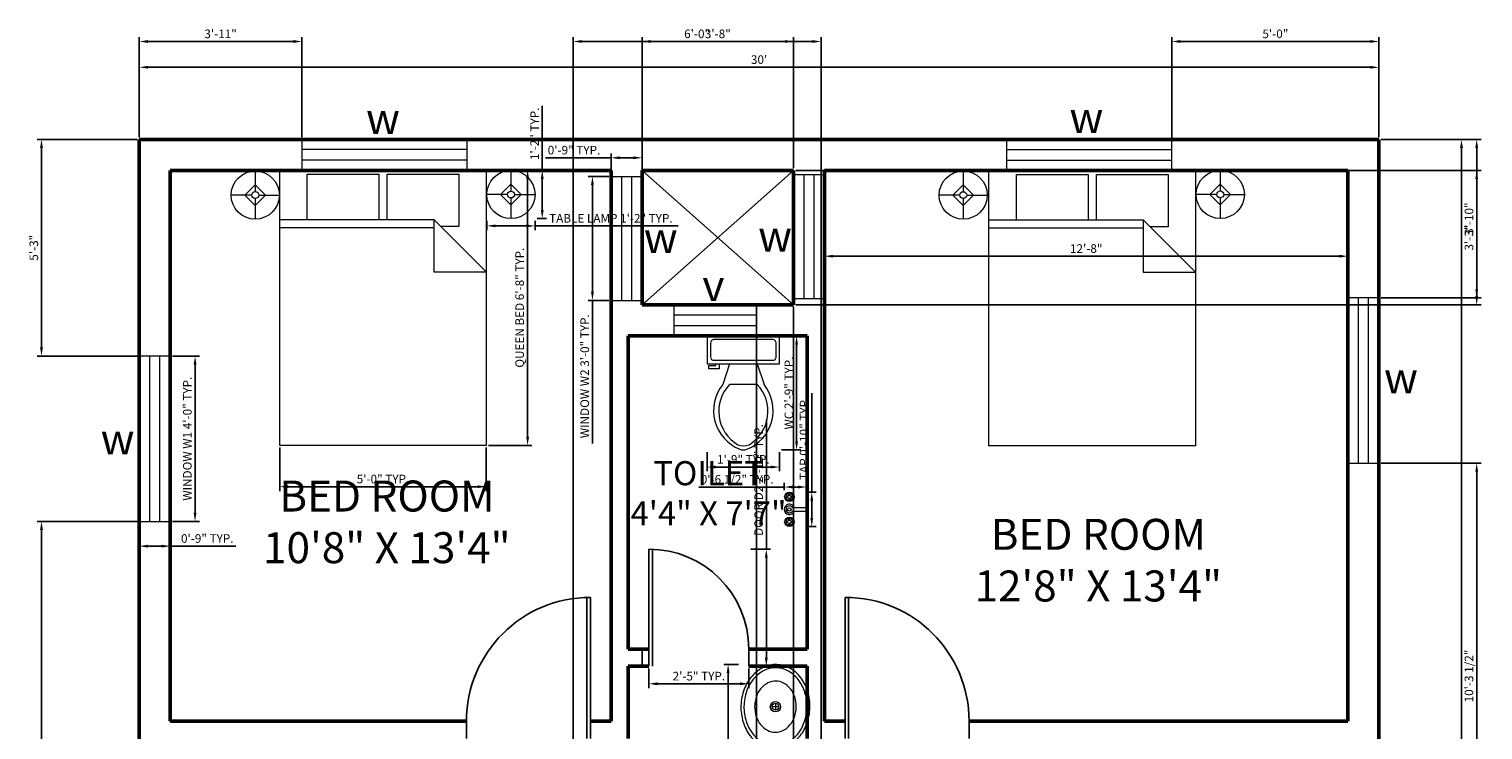
# Model space of a CAD drawing. Units: inches. Extents: x 1962 to 2423, y 2693 to 3296.
# Tile 4 of 4: x 1965 to 2387, y 3092 to 3296. Entities that reach past the tile are written whole.
import ezdxf

# ---------------------------------------------------------------- set-up
doc = ezdxf.new("R2010")
doc.units = ezdxf.units.IN
for name, color, linetype, lineweight in [('A-ANNO-DIMS', 2, 'Continuous', 18), ('A-ANNO-SYMB', 7, 'Continuous', 18), ('A-ANNO-TEXT', 3, 'Continuous', 18), ('A-AREA-IDEN', 7, 'Continuous', 25), ('A-DOOR', 3, 'Continuous', 25), ('A-FLOR-FIXT', 9, 'Continuous', 18), ('A-FURN', 8, 'Continuous', 18), ('A-GLAZ', 4, 'Continuous', 18), ('A-WALL', 7, 'Continuous', 50)]:
    doc.layers.add(name, color=color, linetype=linetype, lineweight=lineweight)
doc.styles.get("Standard").update_dxf_attribs({"font": 'arial.ttf'})
doc.dimstyles.new('ISO-25', dxfattribs={"dimtxt": 2.5, "dimasz": 2.5, "dimexe": 1.25, "dimexo": 0.625, "dimtad": 1, "dimdec": 0, "dimlunit": 3, "dimtxsty": 'Standard', "dimcen": 2.5, "dimadec": 0, "dimazin": 0, "dimtfac": 1, "dimtdec": 0, "dimtmove": 0, "dimatfit": 3, "dimfxl": 1, "dimarcsym": 0})

# ---------------------------------------------------------------- blocks, each defined once
blk = doc.blocks.new('Bed - Queen')
for p, q in [((0, -80.00003), (0, 0)), ((0, 0), (59.99999, 0)), ((59.99999, 0), (59.99999, -80.00003)), ((7.99999, -1.2), (28.79998, -1.2)), ((7.99999, -14.4), (7.99999, -1.2)), ((28.79998, -1.2), (28.79998, -14.4)), ((31.19999, -1.2), (51.99999, -1.2)), ((31.19999, -14.4), (31.19999, -1.2)), ((51.99999, -1.2), (51.99999, -16.4)), ((0, -14.4), (44.8, -14.4)), ((44.8, -16.8), (0, -16.8)), ((59.99999, -29.6), (44.8, -14.4)), ((44.8, -14.4), (44.8, -29.6)), ((51.99999, -16.4), (46.79936, -16.4)), ((44.8, -29.6), (59.99999, -29.6)), ((59.99999, -80.00003), (0, -80.00003))]:
    blk.add_line(p, q)
blk = doc.blocks.new('Lamp - Table')
for p, q in [((0, 7), (0, 1)), ((-1, 0), (-7, 0)), ((0, 3), (-3, 0)), ((-3, 0), (0, -3)), ((3, 0), (0, 3)), ((0, -3), (3, 0)), ((1, 0), (7, 0)), ((0, -1), (0, -7))]:
    blk.add_line(p, q)
for radius in [7, 1]:
    blk.add_circle((0, 0), radius)
blk = doc.blocks.new('Sink - Oval top')
for p, q in [((-1, 0), (1, 0)), ((0, 1), (0, -1))]:
    blk.add_line(p, q)
for points in [[(-12.23, 0.39, 0.117634), (-11.46, -3.36, 0.104469), (-8.88, -6.8, 0.090016), (-5.08, -9.07, 0.08192), (-0.32, -10.02, 0.08192), (4.49, -9.38, 0.090016), (8.42, -7.36, 0.104469), (11.22, -4.09, 0.117634), (12.23, -0.39, 0.117634), (11.46, 3.36, 0.104469), (8.88, 6.8, 0.090016), (5.08, 9.07, 0.08192), (0.32, 10.02, 0.08192), (-4.49, 9.38, 0.090016), (-8.42, 7.36, 0.104469), (-11.22, 4.09, 0.117634)], [(-11.29, 0.16, 0.118622), (-10.52, -3.25, 0.104678), (-8.07, -6.36, 0.089562), (-4.54, -8.37, 0.081185), (-0.13, -9.15, 0.081185), (4.3, -8.49, 0.089562), (7.89, -6.58, 0.104678), (10.42, -3.55, 0.118622), (11.29, -0.16, 0.118622), (10.52, 3.25, 0.104678), (8.07, 6.36, 0.089562), (4.54, 8.37, 0.081185), (0.13, 9.15, 0.081185), (-4.3, 8.49, 0.089562), (-7.89, 6.58, 0.104678), (-10.42, 3.55, 0.118622)], [(-7.42, 0.08, 0.118283), (-6.91, -2.17, 0.104607), (-5.29, -4.21, 0.089718), (-2.97, -5.53, 0.081436), (-0.07, -6.04, 0.081436), (2.84, -5.59, 0.089718), (5.2, -4.33, 0.104607), (6.86, -2.32, 0.118283), (7.42, -0.08, 0.118283), (6.91, 2.17, 0.104607), (5.29, 4.21, 0.089718), (2.97, 5.53, 0.081436), (0.07, 6.04, 0.081436), (-2.84, 5.59, 0.089718), (-5.2, 4.33, 0.104607), (-6.86, 2.32, 0.118283)]]:
    blk.add_lwpolyline(points, format="xyb", close=True)
for radius in [1.5, 1]:
    blk.add_circle((0, 0), radius)
blk = doc.blocks.new('Toilet - top')
for p, q in [((9.5, -6), (9.5, -2)), ((-8, -8.5), (-8, -8)), ((-7, -8), (-7, -9.5)), ((-4, -8), (-6, -14)), ((4, -8), (6, -14)), ((-10, -8.5), (-8, -8.5)), ((-10, -9.5), (-10, -8.5)), ((-7, -9.5), (-10, -9.5)), ((4, -14), (-4, -14))]:
    blk.add_line(p, q)
blk.add_lwpolyline([(10.5, -8), (10.5, 0), (-10.5, 0), (-10.5, -8)], close=True)
for points in [[(-9.5, -2), (-9.5, -6)], [(8.5, -1), (-8.5, -1)], [(-8.5, -7), (8.5, -7)]]:
    blk.add_lwpolyline(points)
for centre, radius, start, end in [((-8.62, -1.88), 0.884, 81.8699, 188.1301), ((8.62, -1.88), 0.884, 351.8699, 98.1301), ((-8.62, -6.12), 0.884, 171.8699, 278.1301), ((8.62, -6.12), 0.884, 261.8699, 8.1301), ((3.52, -21.58), 12.17, 141.4691, 247.9714), ((4.2, -21.82), 11.33, 136.3677, 238.9468), ((-3.52, -21.58), 12.17, 292.0284, 38.5307), ((-4.2, -21.82), 11.33, 301.053, 43.6321), ((0, -27.88), 4, 245.7318, 294.2682), ((0, -29), 4, 254.8605, 285.1395)]:
    blk.add_arc(centre, radius, start, end)
blk = doc.blocks.new('Faucet - Bathroom top')
for p, q in [((-4.107, 0.125), (-4.375, 0.125)), ((-3.75, 0.4788), (-3.75, 0.75)), ((-3.5, 0.482), (-3.5, 0.75)), ((-3.1461, 0.125), (-2.875, 0.125)), ((3.143, 0.125), (2.875, 0.125)), ((3.5, 0.4788), (3.5, 0.75)), ((3.75, 0.482), (3.75, 0.75)), ((4.1039, 0.125), (4.375, 0.125)), ((-4.1039, -0.125), (-4.375, -0.125)), ((-3.75, -0.4821), (-3.75, -0.75)), ((-3.5, -0.4789), (-3.5, -0.75)), ((-3.143, -0.125), (-2.875, -0.125)), ((-0.5, -0.8639), (-0.5, -4.5)), ((0.5, -4.5), (0.5, -0.8631)), ((3.1461, -0.125), (2.875, -0.125)), ((3.5, -0.4821), (3.5, -0.75)), ((3.75, -0.4789), (3.75, -0.75)), ((4.107, -0.125), (4.375, -0.125))]:
    blk.add_line(p, q)
for centre, radius in [((-3.625, 0), 1.375), ((-4.625, 0), 0.2795), ((-3.625, 0), 0.5), ((-3.625, 1), 0.2795), ((-2.625, 0), 0.2795), ((0, 0), 0.5), ((3.625, 0), 1.375), ((2.625, 0), 0.2795), ((3.625, 0), 0.5), ((3.625, 1), 0.2795), ((4.625, 0), 0.2795), ((-3.625, -1), 0.2795), ((3.625, -1), 0.2795)]:
    blk.add_circle(centre, radius)
for centre, radius, start, end in [((-3.625, 0), 1, 105.2407, 164.2093), ((-3.625, 0), 1, 16.44125, 74.07887), ((0, 0), 1.5, 289.6514, 250.3603), ((0, 0), 1, 300.3431, 239.7554), ((3.625, 0), 1, 106.12, 164.0884), ((3.625, 0), 1, 16.23422, 73.90469), ((-3.625, 0), 1, 196.2342, 253.9047), ((-3.625, 0), 1, 286.12, 344.0884), ((3.625, 0), 1, 196.4413, 254.0789), ((3.625, 0), 1, 285.2407, 344.2093), ((0, -4.5), 0.5, 180, 0)]:
    blk.add_arc(centre, radius, start, end)
blk = doc.blocks.new('*D12')
at = {"layer": 'A-ANNO-DIMS', "color": 0, "lineweight": -2, "transparency": 16777216}
for p, q in [((1996.54, 3264.21), (1996.54, 3285.8)), ((2356.54, 3264.21), (2356.54, 3285.8)), ((1999.04, 3284.55), (2354.04, 3284.55))]:
    blk.add_line(p, q, dxfattribs=at)
at = {"layer": 'A-ANNO-DIMS', "color": 0, "transparency": 16777216}
for points in [[(1999.04, 3284.96), (1999.04, 3284.13), (1996.54, 3284.55)], [(2354.04, 3284.96), (2354.04, 3284.13), (2356.54, 3284.55)]]:
    blk.add_solid(points, dxfattribs=at)
at = {"layer": 'Defpoints', "color": 0, "transparency": 16777216}
for p in [(2356.54, 3284.55), (1996.54, 3263.59), (2356.54, 3263.59)]:
    blk.add_point(p, dxfattribs=at)
at = {"layer": 'A-ANNO-DIMS', "color": 0, "transparency": 16777216, "insert": (2176.54, 3286.45), "char_height": 2.5, "attachment_point": 5}
blk.add_mtext("30'", dxfattribs=at)
blk = doc.blocks.new('*D13')
at = {"layer": 'A-ANNO-DIMS', "color": 0, "lineweight": -2, "transparency": 16777216}
for p, q in [((2357.16, 3263.59), (2381.77, 3263.59)), ((2380.52, 3261.09), (2380.52, 2726.09)), ((2357.16, 2723.59), (2381.77, 2723.59))]:
    blk.add_line(p, q, dxfattribs=at)
at = {"layer": 'A-ANNO-DIMS', "color": 0, "transparency": 16777216}
for points in [[(2380.1, 3261.09), (2380.94, 3261.09), (2380.52, 3263.59)], [(2380.1, 2726.09), (2380.94, 2726.09), (2380.52, 2723.59)]]:
    blk.add_solid(points, dxfattribs=at)
at = {"layer": 'Defpoints', "color": 0, "transparency": 16777216}
for p in [(2356.54, 3263.59), (2356.54, 2723.59), (2380.52, 2723.59)]:
    blk.add_point(p, dxfattribs=at)
at = {"layer": 'A-ANNO-DIMS', "color": 0, "transparency": 16777216, "insert": (2378.62, 2993.59), "char_height": 2.5, "attachment_point": 5, "rotation": 90}
blk.add_mtext("45'", dxfattribs=at)
blk = doc.blocks.new('*D14')
at = {"layer": 'A-ANNO-DIMS', "color": 0, "lineweight": -2, "transparency": 16777216}
for p, q in [((2195.54, 3253.96), (2195.54, 3228.43)), ((2347.54, 3253.96), (2347.54, 3228.43)), ((2198.04, 3229.68), (2345.04, 3229.68))]:
    blk.add_line(p, q, dxfattribs=at)
at = {"layer": 'A-ANNO-DIMS', "color": 0, "transparency": 16777216}
for points in [[(2198.04, 3230.09), (2198.04, 3229.26), (2195.54, 3229.68)], [(2345.04, 3230.09), (2345.04, 3229.26), (2347.54, 3229.68)]]:
    blk.add_solid(points, dxfattribs=at)
at = {"layer": 'Defpoints', "color": 0, "transparency": 16777216}
for p in [(2195.54, 3254.59), (2347.54, 3254.59), (2347.54, 3229.68)]:
    blk.add_point(p, dxfattribs=at)
at = {"layer": 'A-ANNO-DIMS', "color": 0, "transparency": 16777216, "insert": (2271.54, 3231.58), "char_height": 2.5, "attachment_point": 5}
blk.add_mtext('12\'-8"', dxfattribs=at)
blk = doc.blocks.new('DOOR-SWING-36IN')
for p, q in [((0, 5), (0, 41)), ((1, 5), (1, 41)), ((0, 5), (0, 0)), ((1, 5), (1, 0)), ((36, 0), (36, 5))]:
    blk.add_line(p, q)
blk.add_arc((0, 5), 36, 0, 90)
blk = doc.blocks.new('DOOR-SWING-29IN')
for p, q in [((0, 5), (0, 34)), ((1, 5), (1, 34)), ((0, 5), (0, 0)), ((1, 5), (1, 0)), ((29, 0), (29, 5))]:
    blk.add_line(p, q)
blk.add_arc((0, 5), 29, 0, 90)
blk = doc.blocks.new('WINDOW-48IN')
for p, q in [((0, 48), (0, 0)), ((9, 48), (0, 48)), ((3, 48), (3, 0)), ((6, 0), (6, 48)), ((9, 0), (9, 48)), ((0, 0), (9, 0))]:
    blk.add_line(p, q)
blk = doc.blocks.new('WINDOW-36IN')
for p, q in [((9, 36), (0, 36)), ((0, 36), (0, 0)), ((3, 36), (3, 0)), ((6, 0), (6, 36)), ((9, 0), (9, 36)), ((9, 0), (0, 0))]:
    blk.add_line(p, q)
blk = doc.blocks.new('VENT-24IN')
for p, q in [((24, 9), (0, 9)), ((0, 9), (0, 0)), ((24, 9), (24, 0)), ((24, 6), (0, 6)), ((0, 3), (24, 3)), ((0, 0), (24, 0))]:
    blk.add_line(p, q)
blk = doc.blocks.new('*D22')
at = {"layer": 'A-ANNO-DIMS', "color": 0, "lineweight": -2, "transparency": 16777216}
for p, q in [((2006.16, 3200.67), (2013.99, 3200.67)), ((2012.74, 3155.17), (2012.74, 3198.17)), ((2006.16, 3152.67), (2013.99, 3152.67))]:
    blk.add_line(p, q, dxfattribs=at)
at = {"layer": 'A-ANNO-DIMS', "color": 0, "transparency": 16777216}
for points in [[(2012.32, 3198.17), (2013.15, 3198.17), (2012.74, 3200.67)], [(2012.32, 3155.17), (2013.15, 3155.17), (2012.74, 3152.67)]]:
    blk.add_solid(points, dxfattribs=at)
at = {"layer": 'Defpoints', "color": 0, "transparency": 16777216}
for p in [(2005.54, 3200.67), (2012.74, 3200.67), (2005.54, 3152.67)]:
    blk.add_point(p, dxfattribs=at)
at = {"layer": 'A-ANNO-DIMS', "color": 0, "transparency": 16777216, "insert": (2010.82, 3176.67), "char_height": 2.5, "attachment_point": 5, "rotation": 90}
blk.add_mtext('WINDOW W1 4\'-0" TYP.', dxfattribs=at)
blk = doc.blocks.new('*D23')
at = {"layer": 'A-ANNO-DIMS', "color": 0, "lineweight": -2, "transparency": 16777216}
for p, q in [((1996.54, 3152.04), (1996.54, 3144.22)), ((2005.54, 3152.04), (2005.54, 3144.22)), ((1999.04, 3145.47), (2003.04, 3145.47)), ((2005.54, 3145.47), (2024.53, 3145.47))]:
    blk.add_line(p, q, dxfattribs=at)
at = {"layer": 'A-ANNO-DIMS', "color": 0, "transparency": 16777216}
for points in [[(1999.04, 3145.88), (1999.04, 3145.05), (1996.54, 3145.47)], [(2003.04, 3145.88), (2003.04, 3145.05), (2005.54, 3145.47)]]:
    blk.add_solid(points, dxfattribs=at)
at = {"layer": 'Defpoints', "color": 0, "transparency": 16777216}
for p in [(1996.54, 3152.67), (2005.54, 3152.67), (2005.54, 3145.47)]:
    blk.add_point(p, dxfattribs=at)
at = {"layer": 'A-ANNO-DIMS', "color": 0, "transparency": 16777216, "insert": (2016.28, 3147.37), "char_height": 2.5, "attachment_point": 5}
blk.add_mtext('0\'-9" TYP.', dxfattribs=at)
blk = doc.blocks.new('*D24')
at = {"layer": 'A-ANNO-DIMS', "color": 0, "lineweight": -2, "transparency": 16777216}
for p, q in [((2097.46, 3239.96), (2097.46, 3237.24)), ((2099.96, 3238.49), (2108.96, 3238.49)), ((2111.46, 3239.96), (2111.46, 3237.24)), ((2111.46, 3238.49), (2153.03, 3238.49))]:
    blk.add_line(p, q, dxfattribs=at)
at = {"layer": 'A-ANNO-DIMS', "color": 0, "transparency": 16777216}
for points in [[(2099.96, 3238.91), (2099.96, 3238.07), (2097.46, 3238.49)], [(2108.96, 3238.91), (2108.96, 3238.07), (2111.46, 3238.49)]]:
    blk.add_solid(points, dxfattribs=at)
at = {"layer": 'Defpoints', "color": 0, "transparency": 16777216}
for p in [(2097.46, 3240.59), (2111.46, 3240.59), (2111.46, 3238.49)]:
    blk.add_point(p, dxfattribs=at)
at = {"layer": 'A-ANNO-DIMS', "color": 0, "transparency": 16777216, "insert": (2133.5, 3240.37), "char_height": 2.5, "attachment_point": 5}
blk.add_mtext('TABLE LAMP 1\'-2" TYP.', dxfattribs=at)
blk = doc.blocks.new('*D25')
at = {"layer": 'A-ANNO-DIMS', "color": 0, "lineweight": -2, "transparency": 16777216}
for p, q in [((2113.56, 3254.59), (2113.56, 3273.34)), ((2112.09, 3254.59), (2114.81, 3254.59)), ((2113.56, 3243.09), (2113.56, 3252.09)), ((2112.09, 3240.59), (2114.81, 3240.59))]:
    blk.add_line(p, q, dxfattribs=at)
at = {"layer": 'A-ANNO-DIMS', "color": 0, "transparency": 16777216}
for points in [[(2113.15, 3252.09), (2113.98, 3252.09), (2113.56, 3254.59)], [(2113.15, 3243.09), (2113.98, 3243.09), (2113.56, 3240.59)]]:
    blk.add_solid(points, dxfattribs=at)
at = {"layer": 'Defpoints', "color": 0, "transparency": 16777216}
for p in [(2111.46, 3254.59), (2113.56, 3254.59), (2111.46, 3240.59)]:
    blk.add_point(p, dxfattribs=at)
at = {"layer": 'A-ANNO-DIMS', "color": 0, "transparency": 16777216, "insert": (2111.68, 3265.22), "char_height": 2.5, "attachment_point": 5, "rotation": 90}
blk.add_mtext('1\'-2" TYP.', dxfattribs=at)
blk = doc.blocks.new('*D28')
at = {"layer": 'A-ANNO-DIMS', "color": 0, "lineweight": -2, "transparency": 16777216}
for p, q in [((2097.94, 3254.73), (2110.56, 3254.73)), ((2109.31, 3177.23), (2109.31, 3252.23)), ((2097.94, 3174.73), (2110.56, 3174.73))]:
    blk.add_line(p, q, dxfattribs=at)
at = {"layer": 'A-ANNO-DIMS', "color": 0, "transparency": 16777216}
for points in [[(2108.9, 3252.23), (2109.73, 3252.23), (2109.31, 3254.73)], [(2108.9, 3177.23), (2109.73, 3177.23), (2109.31, 3174.73)]]:
    blk.add_solid(points, dxfattribs=at)
at = {"layer": 'Defpoints', "color": 0, "transparency": 16777216}
for p in [(2097.31, 3254.73), (2109.31, 3254.73), (2097.31, 3174.73)]:
    blk.add_point(p, dxfattribs=at)
at = {"layer": 'A-ANNO-DIMS', "color": 0, "transparency": 16777216, "insert": (2107.32, 3214.73), "char_height": 2.5, "attachment_point": 5, "rotation": 90}
blk.add_mtext('QUEEN BED 6\'-8" TYP.', dxfattribs=at)
blk = doc.blocks.new('*D29')
at = {"layer": 'A-ANNO-DIMS', "color": 0, "lineweight": -2, "transparency": 16777216}
for p, q in [((2037.31, 3174.11), (2037.31, 3161.48)), ((2097.31, 3174.11), (2097.31, 3161.48)), ((2039.81, 3162.73), (2094.81, 3162.73))]:
    blk.add_line(p, q, dxfattribs=at)
at = {"layer": 'A-ANNO-DIMS', "color": 0, "transparency": 16777216}
for points in [[(2039.81, 3163.15), (2039.81, 3162.32), (2037.31, 3162.73)], [(2094.81, 3163.15), (2094.81, 3162.32), (2097.31, 3162.73)]]:
    blk.add_solid(points, dxfattribs=at)
at = {"layer": 'Defpoints', "color": 0, "transparency": 16777216}
for p in [(2037.31, 3174.73), (2097.31, 3174.73), (2097.31, 3162.73)]:
    blk.add_point(p, dxfattribs=at)
at = {"layer": 'A-ANNO-DIMS', "color": 0, "transparency": 16777216, "insert": (2067.31, 3164.64), "char_height": 2.5, "attachment_point": 5}
blk.add_mtext('5\'-0" TYP.', dxfattribs=at)
blk = doc.blocks.new('*D30')
at = {"layer": 'A-ANNO-DIMS', "color": 0, "lineweight": -2, "transparency": 16777216}
for p, q in [((2178.64, 3144.59), (2178.64, 3182.28)), ((2174.16, 3144.59), (2179.89, 3144.59)), ((2178.64, 3113.09), (2178.64, 3142.09)), ((2174.16, 3110.59), (2179.89, 3110.59))]:
    blk.add_line(p, q, dxfattribs=at)
at = {"layer": 'A-ANNO-DIMS', "color": 0, "transparency": 16777216}
for points in [[(2178.22, 3142.09), (2179.05, 3142.09), (2178.64, 3144.59)], [(2178.22, 3113.09), (2179.05, 3113.09), (2178.64, 3110.59)]]:
    blk.add_solid(points, dxfattribs=at)
at = {"layer": 'Defpoints', "color": 0, "transparency": 16777216}
for p in [(2173.54, 3144.59), (2178.64, 3144.59), (2173.54, 3110.59)]:
    blk.add_point(p, dxfattribs=at)
at = {"layer": 'A-ANNO-DIMS', "color": 0, "transparency": 16777216, "insert": (2176.72, 3164.68), "char_height": 2.5, "attachment_point": 5, "rotation": 90}
blk.add_mtext('DOOR D2 2\'-10" TYP.', dxfattribs=at)
blk = doc.blocks.new('*D31')
at = {"layer": 'A-ANNO-DIMS', "color": 0, "lineweight": -2, "transparency": 16777216}
for p, q in [((2144.54, 3109.96), (2144.54, 3104.24)), ((2173.54, 3109.96), (2173.54, 3104.24)), ((2147.04, 3105.49), (2171.04, 3105.49))]:
    blk.add_line(p, q, dxfattribs=at)
at = {"layer": 'A-ANNO-DIMS', "color": 0, "transparency": 16777216}
for points in [[(2147.04, 3105.91), (2147.04, 3105.07), (2144.54, 3105.49)], [(2171.04, 3105.91), (2171.04, 3105.07), (2173.54, 3105.49)]]:
    blk.add_solid(points, dxfattribs=at)
at = {"layer": 'Defpoints', "color": 0, "transparency": 16777216}
for p in [(2144.54, 3110.59), (2173.54, 3110.59), (2173.54, 3105.49)]:
    blk.add_point(p, dxfattribs=at)
at = {"layer": 'A-ANNO-DIMS', "color": 0, "transparency": 16777216, "insert": (2159.04, 3107.39), "char_height": 2.5, "attachment_point": 5}
blk.add_mtext('2\'-5" TYP.', dxfattribs=at)
blk = doc.blocks.new('*D32')
at = {"layer": 'A-ANNO-DIMS', "color": 0, "lineweight": -2, "transparency": 16777216}
for p, q in [((2183.09, 3206.45), (2188.67, 3206.45)), ((2187.42, 3175.9), (2187.42, 3203.95)), ((2183.09, 3173.4), (2188.67, 3173.4))]:
    blk.add_line(p, q, dxfattribs=at)
at = {"layer": 'A-ANNO-DIMS', "color": 0, "transparency": 16777216}
for points in [[(2187.01, 3203.95), (2187.84, 3203.95), (2187.42, 3206.45)], [(2187.01, 3175.9), (2187.84, 3175.9), (2187.42, 3173.4)]]:
    blk.add_solid(points, dxfattribs=at)
at = {"layer": 'Defpoints', "color": 0, "transparency": 16777216}
for p in [(2182.47, 3206.45), (2187.42, 3206.45), (2182.47, 3173.4)]:
    blk.add_point(p, dxfattribs=at)
at = {"layer": 'A-ANNO-DIMS', "color": 0, "transparency": 16777216, "insert": (2185.51, 3189.93), "char_height": 2.5, "attachment_point": 5, "rotation": 90}
blk.add_mtext('WC 2\'-9" TYP.', dxfattribs=at)
blk = doc.blocks.new('*D33')
at = {"layer": 'A-ANNO-DIMS', "color": 0, "lineweight": -2, "transparency": 16777216}
for p, q in [((2161.47, 3172.78), (2161.47, 3167.2)), ((2182.47, 3172.78), (2182.47, 3167.2)), ((2163.97, 3168.45), (2179.97, 3168.45))]:
    blk.add_line(p, q, dxfattribs=at)
at = {"layer": 'A-ANNO-DIMS', "color": 0, "transparency": 16777216}
for points in [[(2163.97, 3168.86), (2163.97, 3168.03), (2161.47, 3168.45)], [(2179.97, 3168.86), (2179.97, 3168.03), (2182.47, 3168.45)]]:
    blk.add_solid(points, dxfattribs=at)
at = {"layer": 'Defpoints', "color": 0, "transparency": 16777216}
for p in [(2161.47, 3173.4), (2182.47, 3173.4), (2182.47, 3168.45)]:
    blk.add_point(p, dxfattribs=at)
at = {"layer": 'A-ANNO-DIMS', "color": 0, "transparency": 16777216, "insert": (2171.97, 3170.35), "char_height": 2.5, "attachment_point": 5}
blk.add_mtext('1\'-9" TYP.', dxfattribs=at)
blk = doc.blocks.new('*D34')
at = {"layer": 'A-ANNO-DIMS', "color": 0, "lineweight": -2, "transparency": 16777216}
for p, q in [((2191.83, 3161.14), (2191.83, 3189.9)), ((2190.95, 3161.14), (2193.08, 3161.14)), ((2191.83, 3153.64), (2191.83, 3158.64)), ((2190.95, 3151.14), (2193.08, 3151.14))]:
    blk.add_line(p, q, dxfattribs=at)
at = {"layer": 'A-ANNO-DIMS', "color": 0, "transparency": 16777216}
for points in [[(2191.41, 3158.64), (2192.24, 3158.64), (2191.83, 3161.14)], [(2191.41, 3153.64), (2192.24, 3153.64), (2191.83, 3151.14)]]:
    blk.add_solid(points, dxfattribs=at)
at = {"layer": 'Defpoints', "color": 0, "transparency": 16777216}
for p in [(2190.33, 3161.14), (2191.83, 3161.14), (2190.33, 3151.14)]:
    blk.add_point(p, dxfattribs=at)
at = {"layer": 'A-ANNO-DIMS', "color": 0, "transparency": 16777216, "insert": (2189.93, 3176.77), "char_height": 2.5, "attachment_point": 5, "rotation": 90}
blk.add_mtext('TAP 0\'-10" TYP.', dxfattribs=at)
blk = doc.blocks.new('*D35')
at = {"layer": 'A-ANNO-DIMS', "color": 0, "lineweight": -2, "transparency": 16777216}
for p, q in [((2183.83, 3162.64), (2159.01, 3162.64)), ((2183.83, 3161.76), (2183.83, 3163.89)), ((2187.83, 3162.64), (2186.33, 3162.64)), ((2190.33, 3161.76), (2190.33, 3163.89))]:
    blk.add_line(p, q, dxfattribs=at)
at = {"layer": 'A-ANNO-DIMS', "color": 0, "transparency": 16777216}
for points in [[(2186.33, 3163.05), (2186.33, 3162.22), (2183.83, 3162.64)], [(2187.83, 3163.05), (2187.83, 3162.22), (2190.33, 3162.64)]]:
    blk.add_solid(points, dxfattribs=at)
at = {"layer": 'Defpoints', "color": 0, "transparency": 16777216}
for p in [(2183.83, 3162.64), (2183.83, 3161.14), (2190.33, 3161.14)]:
    blk.add_point(p, dxfattribs=at)
at = {"layer": 'A-ANNO-DIMS', "color": 0, "transparency": 16777216, "insert": (2170.17, 3164.56), "char_height": 2.5, "attachment_point": 5}
blk.add_mtext('0\'-6 1/2" TYP.', dxfattribs=at)
blk = doc.blocks.new('*D36')
at = {"layer": 'A-ANNO-DIMS', "color": 0, "lineweight": -2, "transparency": 16777216}
for p, q in [((2132.91, 3252.86), (2126.89, 3252.86)), ((2128.14, 3250.36), (2128.14, 3219.36)), ((2132.91, 3216.86), (2126.89, 3216.86)), ((2128.14, 3216.86), (2128.14, 3175.27))]:
    blk.add_line(p, q, dxfattribs=at)
at = {"layer": 'A-ANNO-DIMS', "color": 0, "transparency": 16777216}
for points in [[(2127.72, 3250.36), (2128.55, 3250.36), (2128.14, 3252.86)], [(2127.72, 3219.36), (2128.55, 3219.36), (2128.14, 3216.86)]]:
    blk.add_solid(points, dxfattribs=at)
at = {"layer": 'Defpoints', "color": 0, "transparency": 16777216}
for p in [(2133.54, 3252.86), (2128.14, 3216.86), (2133.54, 3216.86)]:
    blk.add_point(p, dxfattribs=at)
at = {"layer": 'A-ANNO-DIMS', "color": 0, "transparency": 16777216, "insert": (2126.22, 3194.82), "char_height": 2.5, "attachment_point": 5, "rotation": 90}
blk.add_mtext('WINDOW W2 3\'-0" TYP.', dxfattribs=at)
blk = doc.blocks.new('*D37')
at = {"layer": 'A-ANNO-DIMS', "color": 0, "lineweight": -2, "transparency": 16777216}
for p, q in [((2133.54, 3253.49), (2133.54, 3259.51)), ((2142.54, 3253.49), (2142.54, 3259.51)), ((2133.54, 3258.26), (2114.55, 3258.26)), ((2140.04, 3258.26), (2136.04, 3258.26))]:
    blk.add_line(p, q, dxfattribs=at)
at = {"layer": 'A-ANNO-DIMS', "color": 0, "transparency": 16777216}
for points in [[(2136.04, 3258.68), (2136.04, 3257.85), (2133.54, 3258.26)], [(2140.04, 3258.68), (2140.04, 3257.85), (2142.54, 3258.26)]]:
    blk.add_solid(points, dxfattribs=at)
at = {"layer": 'Defpoints', "color": 0, "transparency": 16777216}
for p in [(2133.54, 3258.26), (2133.54, 3252.86), (2142.54, 3252.86)]:
    blk.add_point(p, dxfattribs=at)
at = {"layer": 'A-ANNO-DIMS', "color": 0, "transparency": 16777216, "insert": (2122.79, 3260.16), "char_height": 2.5, "attachment_point": 5}
blk.add_mtext('0\'-9" TYP.', dxfattribs=at)
blk = doc.blocks.new('*D48')
at = {"layer": 'A-ANNO-DIMS', "color": 0, "lineweight": -2, "transparency": 16777216}
for p, q in [((2170.6, 3111.12), (2166.29, 3111.12)), ((2167.54, 3108.62), (2167.54, 3089.07)), ((2170.6, 3086.57), (2166.29, 3086.57)), ((2167.54, 3086.57), (2167.54, 3059.01))]:
    blk.add_line(p, q, dxfattribs=at)
at = {"layer": 'A-ANNO-DIMS', "color": 0, "transparency": 16777216}
for points in [[(2167.12, 3108.62), (2167.96, 3108.62), (2167.54, 3111.12)], [(2167.12, 3089.07), (2167.96, 3089.07), (2167.54, 3086.57)]]:
    blk.add_solid(points, dxfattribs=at)
at = {"layer": 'Defpoints', "color": 0, "transparency": 16777216}
for p in [(2171.22, 3111.12), (2167.54, 3086.57), (2171.22, 3086.57)]:
    blk.add_point(p, dxfattribs=at)
at = {"layer": 'A-ANNO-DIMS', "color": 0, "transparency": 16777216, "insert": (2165.62, 3071.54), "char_height": 2.5, "attachment_point": 5, "rotation": 90}
blk.add_mtext('BASIN 2\'-0 1/2"', dxfattribs=at)
blk = doc.blocks.new('*D53')
at = {"layer": 'A-ANNO-DIMS', "color": 0, "lineweight": -2, "transparency": 16777216}
for p, q in [((2122.54, 2989.21), (2122.54, 3293.29)), ((2194.54, 2989.21), (2194.54, 3293.29)), ((2125.04, 3292.04), (2192.04, 3292.04))]:
    blk.add_line(p, q, dxfattribs=at)
at = {"layer": 'A-ANNO-DIMS', "color": 0, "transparency": 16777216}
for points in [[(2125.04, 3292.46), (2125.04, 3291.63), (2122.54, 3292.04)], [(2192.04, 3292.46), (2192.04, 3291.63), (2194.54, 3292.04)]]:
    blk.add_solid(points, dxfattribs=at)
at = {"layer": 'Defpoints', "color": 0, "transparency": 16777216}
for p in [(2194.54, 3292.04), (2122.54, 2988.59), (2194.54, 2988.59)]:
    blk.add_point(p, dxfattribs=at)
at = {"layer": 'A-ANNO-DIMS', "color": 0, "transparency": 16777216, "insert": (2158.54, 3293.94), "char_height": 2.5, "attachment_point": 5}
blk.add_mtext('6\'-0"', dxfattribs=at)
blk = doc.blocks.new('*D54')
at = {"layer": 'A-ANNO-DIMS', "color": 0, "lineweight": -2, "transparency": 16777216}
for p, q in [((2142.54, 3255.21), (2142.54, 3293.29)), ((2186.54, 3255.21), (2186.54, 3293.29)), ((2145.04, 3292.04), (2184.04, 3292.04))]:
    blk.add_line(p, q, dxfattribs=at)
at = {"layer": 'A-ANNO-DIMS', "color": 0, "transparency": 16777216}
for points in [[(2145.04, 3292.46), (2145.04, 3291.63), (2142.54, 3292.04)], [(2184.04, 3292.46), (2184.04, 3291.63), (2186.54, 3292.04)]]:
    blk.add_solid(points, dxfattribs=at)
at = {"layer": 'Defpoints', "color": 0, "transparency": 16777216}
for p in [(2186.54, 3292.04), (2142.54, 3254.59), (2186.54, 3254.59)]:
    blk.add_point(p, dxfattribs=at)
at = {"layer": 'A-ANNO-DIMS', "color": 0, "transparency": 16777216, "insert": (2164.54, 3293.94), "char_height": 2.5, "attachment_point": 5}
blk.add_mtext('3\'-8"', dxfattribs=at)
blk = doc.blocks.new('*D55')
at = {"layer": 'A-ANNO-DIMS', "color": 0, "lineweight": -2, "transparency": 16777216}
for p, q in [((2187.16, 3254.59), (2386.19, 3254.59)), ((2384.94, 3218.09), (2384.94, 3252.09)), ((2187.16, 3215.59), (2386.19, 3215.59))]:
    blk.add_line(p, q, dxfattribs=at)
at = {"layer": 'A-ANNO-DIMS', "color": 0, "transparency": 16777216}
for points in [[(2384.52, 3252.09), (2385.35, 3252.09), (2384.94, 3254.59)], [(2384.52, 3218.09), (2385.35, 3218.09), (2384.94, 3215.59)]]:
    blk.add_solid(points, dxfattribs=at)
at = {"layer": 'Defpoints', "color": 0, "transparency": 16777216}
for p in [(2186.54, 3254.59), (2384.94, 3254.59), (2186.54, 3215.59)]:
    blk.add_point(p, dxfattribs=at)
at = {"layer": 'A-ANNO-DIMS', "color": 0, "transparency": 16777216, "insert": (2383.03, 3235.09), "char_height": 2.5, "attachment_point": 5, "rotation": 90}
blk.add_mtext('3\'-3"', dxfattribs=at)
blk = doc.blocks.new('*D56')
at = {"layer": 'A-ANNO-DIMS', "color": 0, "lineweight": -2, "transparency": 16777216}
for p, q in [((1996.54, 3264.21), (1996.54, 3293.29)), ((2043.78, 3264.27), (2043.78, 3293.29)), ((1999.04, 3292.04), (2041.28, 3292.04))]:
    blk.add_line(p, q, dxfattribs=at)
at = {"layer": 'A-ANNO-DIMS', "color": 0, "transparency": 16777216}
for points in [[(1999.04, 3292.46), (1999.04, 3291.63), (1996.54, 3292.04)], [(2041.28, 3292.46), (2041.28, 3291.63), (2043.78, 3292.04)]]:
    blk.add_solid(points, dxfattribs=at)
at = {"layer": 'Defpoints', "color": 0, "transparency": 16777216}
for p in [(2043.78, 3292.04), (1996.54, 3263.59), (2043.78, 3263.64)]:
    blk.add_point(p, dxfattribs=at)
at = {"layer": 'A-ANNO-DIMS', "color": 0, "transparency": 16777216, "insert": (2020.16, 3293.94), "char_height": 2.5, "attachment_point": 5}
blk.add_mtext('3\'-11"', dxfattribs=at)
blk = doc.blocks.new('*D57')
at = {"layer": 'A-ANNO-DIMS', "color": 0, "lineweight": -2, "transparency": 16777216}
for p, q in [((2296.4, 3264.17), (2296.4, 3293.29)), ((2356.54, 3264.21), (2356.54, 3293.29)), ((2298.9, 3292.04), (2354.04, 3292.04))]:
    blk.add_line(p, q, dxfattribs=at)
at = {"layer": 'A-ANNO-DIMS', "color": 0, "transparency": 16777216}
for points in [[(2298.9, 3292.46), (2298.9, 3291.63), (2296.4, 3292.04)], [(2354.04, 3292.46), (2354.04, 3291.63), (2356.54, 3292.04)]]:
    blk.add_solid(points, dxfattribs=at)
at = {"layer": 'Defpoints', "color": 0, "transparency": 16777216}
for p in [(2356.54, 3292.04), (2296.4, 3263.55), (2356.54, 3263.59)]:
    blk.add_point(p, dxfattribs=at)
at = {"layer": 'A-ANNO-DIMS', "color": 0, "transparency": 16777216, "insert": (2326.47, 3293.94), "char_height": 2.5, "attachment_point": 5}
blk.add_mtext('5\'-0"', dxfattribs=at)
blk = doc.blocks.new('*D58')
at = {"layer": 'A-ANNO-DIMS', "color": 0, "lineweight": -2, "transparency": 16777216}
for p, q in [((1995.91, 3263.59), (1966.89, 3263.59)), ((1968.14, 3203.17), (1968.14, 3261.09)), ((1995.91, 3200.67), (1966.89, 3200.67))]:
    blk.add_line(p, q, dxfattribs=at)
at = {"layer": 'A-ANNO-DIMS', "color": 0, "transparency": 16777216}
for points in [[(1967.72, 3261.09), (1968.55, 3261.09), (1968.14, 3263.59)], [(1967.72, 3203.17), (1968.55, 3203.17), (1968.14, 3200.67)]]:
    blk.add_solid(points, dxfattribs=at)
at = {"layer": 'Defpoints', "color": 0, "transparency": 16777216}
for p in [(1968.14, 3263.59), (1996.54, 3263.59), (1996.54, 3200.67)]:
    blk.add_point(p, dxfattribs=at)
at = {"layer": 'A-ANNO-DIMS', "color": 0, "transparency": 16777216, "insert": (1966.23, 3232.13), "char_height": 2.5, "attachment_point": 5, "rotation": 90}
blk.add_mtext('5\'-3"', dxfattribs=at)
blk = doc.blocks.new('*D59')
at = {"layer": 'A-ANNO-DIMS', "color": 0, "lineweight": -2, "transparency": 16777216}
for p, q in [((2357.16, 3263.59), (2386.19, 3263.59)), ((2384.94, 3220.08), (2384.94, 3261.09)), ((2357.16, 3217.58), (2386.19, 3217.58))]:
    blk.add_line(p, q, dxfattribs=at)
at = {"layer": 'A-ANNO-DIMS', "color": 0, "transparency": 16777216}
for points in [[(2384.52, 3261.09), (2385.35, 3261.09), (2384.94, 3263.59)], [(2384.52, 3220.08), (2385.35, 3220.08), (2384.94, 3217.58)]]:
    blk.add_solid(points, dxfattribs=at)
at = {"layer": 'Defpoints', "color": 0, "transparency": 16777216}
for p in [(2356.54, 3263.59), (2384.94, 3263.59), (2356.54, 3217.58)]:
    blk.add_point(p, dxfattribs=at)
at = {"layer": 'A-ANNO-DIMS', "color": 0, "transparency": 16777216, "insert": (2383.03, 3240.58), "char_height": 2.5, "attachment_point": 5, "rotation": 90}
blk.add_mtext('3\'-10"', dxfattribs=at)
blk = doc.blocks.new('*D60')
at = {"layer": 'A-ANNO-DIMS', "color": 0, "lineweight": -2, "transparency": 16777216}
for p, q in [((2357.16, 3169.58), (2386.19, 3169.58)), ((2384.94, 3048.42), (2384.94, 3167.08)), ((2357.16, 3045.92), (2386.19, 3045.92))]:
    blk.add_line(p, q, dxfattribs=at)
at = {"layer": 'A-ANNO-DIMS', "color": 0, "transparency": 16777216}
for points in [[(2384.52, 3167.08), (2385.35, 3167.08), (2384.94, 3169.58)], [(2384.52, 3048.42), (2385.35, 3048.42), (2384.94, 3045.92)]]:
    blk.add_solid(points, dxfattribs=at)
at = {"layer": 'Defpoints', "color": 0, "transparency": 16777216}
for p in [(2356.54, 3169.58), (2384.94, 3169.58), (2356.54, 3045.92)]:
    blk.add_point(p, dxfattribs=at)
at = {"layer": 'A-ANNO-DIMS', "color": 0, "transparency": 16777216, "insert": (2383.02, 3107.75), "char_height": 2.5, "attachment_point": 5, "rotation": 90}
blk.add_mtext('10\'-3 1/2"', dxfattribs=at)
blk = doc.blocks.new('*D63')
at = {"layer": 'A-ANNO-DIMS', "color": 0, "lineweight": -2, "transparency": 16777216}
for p, q in [((1995.91, 3152.67), (1966.89, 3152.67)), ((1968.14, 2964.06), (1968.14, 3150.17)), ((1995.91, 2961.56), (1966.89, 2961.56))]:
    blk.add_line(p, q, dxfattribs=at)
at = {"layer": 'A-ANNO-DIMS', "color": 0, "transparency": 16777216}
for points in [[(1967.72, 3150.17), (1968.55, 3150.17), (1968.14, 3152.67)], [(1967.72, 2964.06), (1968.55, 2964.06), (1968.14, 2961.56)]]:
    blk.add_solid(points, dxfattribs=at)
at = {"layer": 'Defpoints', "color": 0, "transparency": 16777216}
for p in [(1968.14, 3152.67), (1996.54, 3152.67), (1996.54, 2961.56)]:
    blk.add_point(p, dxfattribs=at)
at = {"layer": 'A-ANNO-DIMS', "color": 0, "transparency": 16777216, "insert": (1966.24, 3057.11), "char_height": 2.5, "attachment_point": 5, "rotation": 90}
blk.add_mtext('15\'-11"', dxfattribs=at)
blk = doc.blocks.new('*D71')
at = {"layer": 'A-ANNO-DIMS', "color": 0, "lineweight": -2, "transparency": 16777216}
for p, q in [((2175.74, 3214.96), (2175.74, 2693.94)), ((2186.54, 3214.96), (2186.54, 2693.94)), ((2184.04, 2695.19), (2178.24, 2695.19))]:
    blk.add_line(p, q, dxfattribs=at)
at = {"layer": 'A-ANNO-DIMS', "color": 0, "transparency": 16777216}
for points in [[(2178.24, 2695.61), (2178.24, 2694.77), (2175.74, 2695.19)], [(2184.04, 2695.61), (2184.04, 2694.77), (2186.54, 2695.19)]]:
    blk.add_solid(points, dxfattribs=at)
at = {"layer": 'Defpoints', "color": 0, "transparency": 16777216}
for p in [(2175.74, 3215.59), (2186.54, 3215.59), (2175.74, 2695.19)]:
    blk.add_point(p, dxfattribs=at)
at = {"layer": 'A-ANNO-DIMS', "color": 0, "transparency": 16777216, "insert": (2181.14, 2697.09), "char_height": 2.5, "attachment_point": 5}
blk.add_mtext('0\'-11"', dxfattribs=at)

msp = doc.modelspace()

# ---------------------------------------------------------------- linework, layer by layer
at = {"layer": 'A-ANNO-SYMB'}
for p, q in [((2142.54, 3254.59), (2186.54, 3215.59)), ((2186.54, 3254.59), (2142.54, 3215.59))]:
    msp.add_line(p, q, dxfattribs=at)
at = {"layer": 'A-DOOR'}
msp.add_line((2142.54, 3115.59), (2142.54, 3110.59), dxfattribs=at)
at = {"layer": 'A-WALL'}
for p, q in [((1996.54, 3263.59), (1996.54, 2723.59)), ((2356.54, 3263.59), (1996.54, 3263.59)), ((2356.54, 2723.59), (2356.54, 3263.59)), ((2005.54, 3254.59), (2005.54, 3094.59)), ((2133.54, 3254.59), (2005.54, 3254.59)), ((2133.54, 3254.59), (2133.54, 3094.59)), ((2186.54, 3254.59), (2142.54, 3254.59)), ((2142.54, 3254.59), (2142.54, 3215.59)), ((2186.54, 3215.59), (2186.54, 3254.59)), ((2186.54, 3215.59), (2186.54, 3254.59)), ((2347.54, 3254.59), (2195.54, 3254.59)), ((2195.54, 3094.59), (2195.54, 3254.59)), ((2347.54, 3094.59), (2347.54, 3254.59)), ((2186.54, 3215.59), (2142.54, 3215.59)), ((2190.54, 3206.59), (2138.54, 3206.59)), ((2138.54, 3206.59), (2138.54, 3115.59)), ((2190.54, 3115.59), (2190.54, 3206.59)), ((2138.54, 3115.59), (2144.54, 3115.59)), ((2144.54, 3115.59), (2138.54, 3115.59)), ((2190.54, 3115.59), (2173.54, 3115.59)), ((2138.54, 3110.59), (2138.54, 3089.59)), ((2144.54, 3110.59), (2138.54, 3110.59)), ((2190.54, 3110.59), (2173.54, 3110.59)), ((2190.54, 3110.59), (2184.54, 3110.59)), ((2190.54, 3089.59), (2190.54, 3110.59)), ((2091.54, 3094.59), (2005.54, 3094.59)), ((2133.54, 3094.59), (2127.54, 3094.59)), ((2133.54, 3094.59), (2127.54, 3094.59)), ((2195.54, 3094.59), (2201.54, 3094.59)), ((2201.54, 3094.59), (2195.54, 3094.59)), ((2347.54, 3094.59), (2237.54, 3094.59))]:
    msp.add_line(p, q, dxfattribs=at)

# ---------------------------------------------------------------- block references
at = {"layer": 'A-DOOR'}
for name, p in [('DOOR-SWING-29IN', (2144.54, 3110.59)), ('DOOR-SWING-36IN', (2201.54, 3089.59))]:
    msp.add_blockref(name, p, dxfattribs=at)
at = {"layer": 'A-DOOR', "extrusion": (0, 0, -1), "zscale": -1}
msp.add_blockref('DOOR-SWING-36IN', (-2127.54, 3089.59), dxfattribs=at)
at = {"layer": 'A-FLOR-FIXT'}
msp.add_blockref('Toilet - top', (2171.97, 3206.45), dxfattribs=at)
for name, p, rotation in [('Faucet - Bathroom top', (2185.33, 3156.14), 90), ('Sink - Oval top', (2181.29, 3098.84), 270)]:
    msp.add_blockref(name, p, dxfattribs=dict(at, rotation=rotation))
at = {"layer": 'A-FURN'}
for name, p in [('Lamp - Table', (2030.22, 3247.43)), ('Bed - Queen', (2037.31, 3254.73)), ('Lamp - Table', (2104.46, 3247.59)), ('Lamp - Table', (2235.82, 3247.42)), ('Bed - Queen', (2243.29, 3254.64)), ('Lamp - Table', (2310.47, 3247.62))]:
    msp.add_blockref(name, p, dxfattribs=at)
at = {"layer": 'A-GLAZ'}
for name, p, rotation in [('WINDOW-48IN', (2043.78, 3263.64), 270.0000000000009), ('WINDOW-48IN', (2248.4, 3263.55), 269.9999999999984), ('WINDOW-36IN', (2142.54, 3252.86), 180)]:
    msp.add_blockref(name, p, dxfattribs=dict(at, rotation=rotation))
for name, p in [('WINDOW-36IN', (2186.54, 3217.3)), ('WINDOW-48IN', (2347.54, 3169.58)), ('VENT-24IN', (2151.74, 3206.59)), ('WINDOW-48IN', (1996.54, 3152.67))]:
    msp.add_blockref(name, p, dxfattribs=at)

# ---------------------------------------------------------------- texts
at = {"layer": 'A-ANNO-TEXT', "char_height": 9, "attachment_point": 1}
for s, width, insert in [('\\pxqc;w', 21.5056, (2056.55, 3274.22)), ('\\pxqc;w', 21.5056, (2260.83, 3274.48)), ('\\pxqc;w', 21.5056, (2137.22, 3239.57)), ('\\pxqc;w', 21.5056, (2170.42, 3240.02)), ('\\pxqc;v', 24.7086, (2150.92, 3225.65)), ('\\pxqc;w', 21.5056, (2352.19, 3198.86)), ('\\pxqc;w', 21.5056, (1979.48, 3181.09))]:
    msp.add_mtext_dynamic_manual_height_columns(s, width=width, gutter_width=12.5, heights=[0], dxfattribs=dict(at, insert=insert))
at = {"layer": 'A-AREA-IDEN', "attachment_point": 1}
for s, insert, char_height in [('\\pxqc;TOILET\\P4\'4" X 7\'7"', (2110.92, 3170.15), 7), ('\\pxqc;BED ROOM \\P10\'8" X 13\'4"', (2017.5, 3164.52), 9), ('\\pxqc;BED ROOM\\P12\'8" X 13\'4" ', (2224.11, 3153.4), 9)]:
    msp.add_mtext_dynamic_manual_height_columns(s, width=101.8726, gutter_width=12.5, heights=[0], dxfattribs=dict(at, insert=insert, char_height=char_height))

# ---------------------------------------------------------------- dimensions: what is measured, and where the dimension line sits
at = {"layer": 'A-ANNO-DIMS'}
for base, p1, p2, override, picture, middle in [((2043.78, 3292.04), (1996.54, 3263.59), (2043.78, 3263.64), {"dimdec": 1, "dimlfac": 1, "dimrnd": 0, "dimzin": 1, "dimdsep": 46, "dimlunit": 4, "dimfrac": 2}, '*D56', (2020.16, 3293.94)), ((2194.54, 3292.04), (2122.54, 2988.59), (2194.54, 2988.59), {"dimdec": 1, "dimlfac": 1, "dimrnd": 0, "dimzin": 1, "dimdsep": 46, "dimlunit": 4, "dimfrac": 2}, '*D53', (2158.54, 3293.94)), ((2186.54, 3292.04), (2142.54, 3254.59), (2186.54, 3254.59), {"dimdec": 1, "dimlfac": 1, "dimrnd": 0, "dimzin": 1, "dimdsep": 46, "dimlunit": 4, "dimfrac": 2}, '*D54', (2164.54, 3293.94)), ((2356.54, 3292.04), (2296.4, 3263.55), (2356.54, 3263.59), {"dimdec": 1, "dimlfac": 1, "dimrnd": 0, "dimzin": 1, "dimdsep": 46, "dimlunit": 4, "dimfrac": 2}, '*D57', (2326.47, 3293.94)), ((2356.54, 3284.55), (1996.54, 3263.59), (2356.54, 3263.59), {"dimclrd": 0, "dimclre": 0, "dimclrt": 0}, '*D12', (2176.54, 3286.45)), ((2347.54, 3229.68), (2195.54, 3254.59), (2347.54, 3254.59), {"dimclrd": 0, "dimclre": 0, "dimclrt": 0}, '*D14', (2271.54, 3231.58)), ((2175.74, 2695.19), (2186.54, 3215.59), (2175.74, 3215.59), {"dimdec": 1, "dimlfac": 1, "dimrnd": 0, "dimzin": 1, "dimdsep": 46, "dimlunit": 4, "dimfrac": 2}, '*D71', (2181.14, 2697.09))]:
    dim = msp.add_linear_dim(base=base, p1=p1, p2=p2, dimstyle='ISO-25', override=override, dxfattribs=at)
    dim.commit()
    dim.dimension.update_dxf_attribs({"geometry": picture, "text_midpoint": middle})
for base, p1, p2, angle, text, picture, middle in [((2113.56, 3254.59), (2111.46, 3240.59), (2111.46, 3254.59), 90, '<> TYP.', '*D25', (2111.68, 3265.22)), ((2133.54, 3258.26), (2142.54, 3252.86), (2133.54, 3252.86), 180, '<> TYP.', '*D37', (2122.79, 3260.16)), ((2109.31, 3254.73), (2097.31, 3174.73), (2097.31, 3254.73), 90, 'QUEEN BED <> TYP.', '*D28', (2107.32, 3214.73)), ((2128.14, 3216.86), (2133.54, 3252.86), (2133.54, 3216.86), 270, 'WINDOW W2 <> TYP.', '*D36', (2126.22, 3194.82)), ((2187.4228, 3206.4497), (2182.4659, 3173.4034), (2182.4659, 3206.4497), 90, 'WC <> TYP.', '*D32', (2185.5052, 3189.9266)), ((2012.74, 3200.67), (2005.54, 3152.67), (2005.54, 3200.67), 90, 'WINDOW W1 <> TYP.', '*D22', (2010.82, 3176.67)), ((2191.83, 3161.14), (2190.33, 3151.14), (2190.33, 3161.14), 90, 'TAP <> TYP.', '*D34', (2189.93, 3176.77)), ((2178.64, 3144.59), (2173.54, 3110.59), (2173.54, 3144.59), 90, 'DOOR D2 <> TYP.', '*D30', (2176.72, 3164.68)), ((2183.83, 3162.64), (2190.33, 3161.14), (2183.83, 3161.14), 180, '<> TYP.', '*D35', (2170.17, 3164.56)), ((2167.5395, 3086.5685), (2171.2221, 3111.1193), (2171.2221, 3086.5685), 270, 'BASIN <>', '*D48', (2165.6218, 3071.5378))]:
    dim = msp.add_linear_dim(base=base, p1=p1, p2=p2, angle=angle, text=text, dimstyle='ISO-25', override={"dimdec": 1, "dimlfac": 1, "dimrnd": 0, "dimzin": 1, "dimdsep": 46, "dimlunit": 4, "dimfrac": 2}, dxfattribs=at)
    dim.commit()
    dim.dimension.update_dxf_attribs({"geometry": picture, "text_midpoint": middle})
for base, p1, p2, override, picture, middle in [((1968.14, 3263.59), (1996.54, 3200.67), (1996.54, 3263.59), {"dimdec": 1, "dimlfac": 1, "dimrnd": 0, "dimzin": 1, "dimdsep": 46, "dimlunit": 4, "dimfrac": 2}, '*D58', (1966.23, 3232.13)), ((2380.52, 2723.59), (2356.54, 3263.59), (2356.54, 2723.59), {"dimclrd": 0, "dimclre": 0, "dimclrt": 0}, '*D13', (2378.62, 2993.59)), ((2384.94, 3263.59), (2356.54, 3217.58), (2356.54, 3263.59), {"dimdec": 1, "dimlfac": 1, "dimrnd": 0, "dimzin": 1, "dimdsep": 46, "dimlunit": 4, "dimfrac": 2}, '*D59', (2383.03, 3240.58)), ((2384.94, 3254.59), (2186.54, 3215.59), (2186.54, 3254.59), {"dimdec": 1, "dimlfac": 1, "dimrnd": 0, "dimzin": 1, "dimdsep": 46, "dimlunit": 4, "dimfrac": 2}, '*D55', (2383.03, 3235.09)), ((2384.94, 3169.58), (2356.54, 3045.92), (2356.54, 3169.58), {"dimdec": 1, "dimlfac": 1, "dimrnd": 0, "dimzin": 1, "dimdsep": 46, "dimlunit": 4, "dimfrac": 2}, '*D60', (2383.02, 3107.75)), ((1968.14, 3152.67), (1996.54, 2961.56), (1996.54, 3152.67), {"dimdec": 1, "dimlfac": 1, "dimrnd": 0, "dimzin": 1, "dimdsep": 46, "dimlunit": 4, "dimfrac": 2}, '*D63', (1966.24, 3057.11))]:
    dim = msp.add_linear_dim(base=base, p1=p1, p2=p2, angle=90, dimstyle='ISO-25', override=override, dxfattribs=at)
    dim.commit()
    dim.dimension.update_dxf_attribs({"geometry": picture, "text_midpoint": middle})
for base, p1, p2, text, picture, middle in [((2111.46, 3238.49), (2097.46, 3240.59), (2111.46, 3240.59), 'TABLE LAMP <> TYP.', '*D24', (2133.5, 3240.37)), ((2097.31, 3162.73), (2037.31, 3174.73), (2097.31, 3174.73), '<> TYP.', '*D29', (2067.31, 3164.64)), ((2182.47, 3168.45), (2161.47, 3173.4), (2182.47, 3173.4), '<> TYP.', '*D33', (2171.97, 3170.35)), ((2005.54, 3145.47), (1996.54, 3152.67), (2005.54, 3152.67), '<> TYP.', '*D23', (2016.28, 3147.37)), ((2173.54, 3105.49), (2144.54, 3110.59), (2173.54, 3110.59), '<> TYP.', '*D31', (2159.04, 3107.39))]:
    dim = msp.add_linear_dim(base=base, p1=p1, p2=p2, text=text, dimstyle='ISO-25', override={"dimdec": 1, "dimlfac": 1, "dimrnd": 0, "dimzin": 1, "dimdsep": 46, "dimlunit": 4, "dimfrac": 2}, dxfattribs=at)
    dim.commit()
    dim.dimension.update_dxf_attribs({"geometry": picture, "text_midpoint": middle})

doc.saveas('drawing.dxf')
